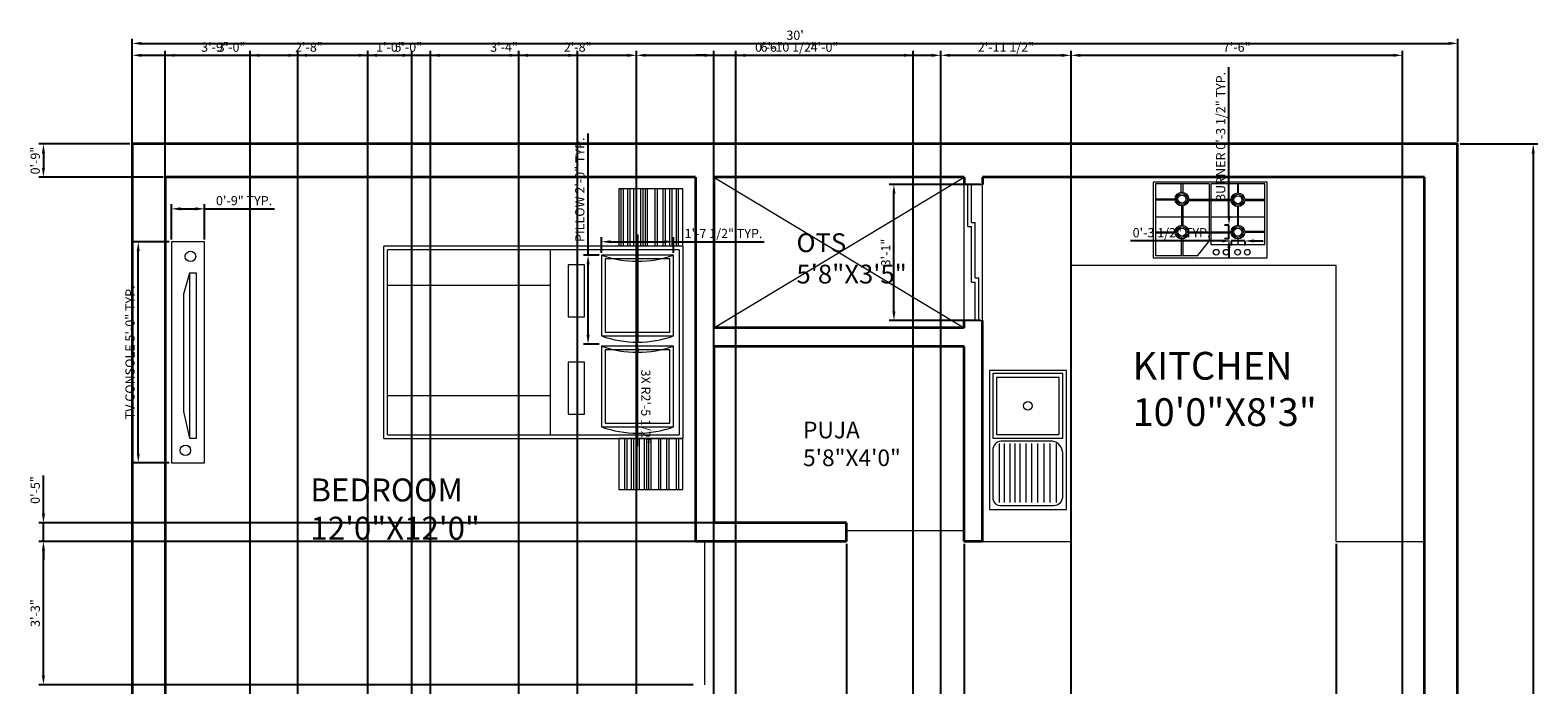
# Model space of a CAD drawing. Units: inches. Extents: x 364 to 777, y 253 to 730.
# Tile 2 of 2: x 364 to 773, y 552 to 730. Entities that reach past the tile are written whole.
import ezdxf

# ---------------------------------------------------------------- set-up
doc = ezdxf.new("R2010")
doc.units = ezdxf.units.IN
for name, color, linetype, lineweight in [('A-ANNO-DIMS', 2, 'Continuous', 18), ('A-AREA-IDEN', 7, 'Continuous', 25), ('A-DOOR', 4, 'Continuous', 18), ('A-EQPM', 8, 'Continuous', 18), ('A-FLOR-CASE', 8, 'Continuous', 18), ('A-FLOR-FIXT', 8, 'Continuous', 18), ('A-FLOR-OPEN', 8, 'Continuous', 13), ('A-FURN', 8, 'Continuous', 18), ('A-GLAZ', 5, 'Continuous', 18), ('A-WALL', 7, 'Continuous', 35)]:
    doc.layers.add(name, color=color, linetype=linetype, lineweight=lineweight)
doc.styles.get("Standard").update_dxf_attribs({"font": 'arial.ttf'})
doc.dimstyles.new('ISO-25', dxfattribs={"dimtxt": 2.5, "dimasz": 2.5, "dimexe": 1.25, "dimexo": 0.625, "dimtad": 1, "dimdec": 0, "dimlunit": 3, "dimtxsty": 'Standard', "dimcen": 2.5, "dimadec": 0, "dimazin": 0, "dimtfac": 1, "dimtdec": 0, "dimtmove": 0, "dimatfit": 3, "dimfxl": 1, "dimarcsym": 0})

# ---------------------------------------------------------------- blocks, each defined once
blk = doc.blocks.new('*D1')
at = {"layer": 'A-ANNO-DIMS', "color": 0, "lineweight": -2, "transparency": 16777216}
for p, q in [((752.34, 699.12), (773.4, 699.12)), ((772.15, 696.62), (772.15, 341.62)), ((752.34, 339.12), (773.4, 339.12))]:
    blk.add_line(p, q, dxfattribs=at)
at = {"layer": 'A-ANNO-DIMS', "color": 0, "transparency": 16777216}
for points in [[(771.73, 696.62), (772.57, 696.62), (772.15, 699.12)], [(771.73, 341.62), (772.57, 341.62), (772.15, 339.12)]]:
    blk.add_solid(points, dxfattribs=at)
at = {"layer": 'Defpoints', "color": 0, "transparency": 16777216}
for p in [(751.71, 699.12), (751.71, 339.12), (772.15, 339.12)]:
    blk.add_point(p, dxfattribs=at)
at = {"layer": 'A-ANNO-DIMS', "color": 0, "transparency": 16777216, "insert": (770.25, 519.12), "char_height": 2.5, "attachment_point": 5, "rotation": 90}
blk.add_mtext("30'", dxfattribs=at)
blk = doc.blocks.new('*D2')
at = {"layer": 'A-ANNO-DIMS', "color": 0, "lineweight": -2, "transparency": 16777216}
for p, q in [((391.61, 699.74), (391.61, 727.71)), ((394.11, 726.46), (749.21, 726.46)), ((751.71, 699.74), (751.71, 727.71))]:
    blk.add_line(p, q, dxfattribs=at)
at = {"layer": 'A-ANNO-DIMS', "color": 0, "transparency": 16777216}
for points in [[(394.11, 726.88), (394.11, 726.04), (391.61, 726.46)], [(749.21, 726.88), (749.21, 726.04), (751.71, 726.46)]]:
    blk.add_solid(points, dxfattribs=at)
at = {"layer": 'Defpoints', "color": 0, "transparency": 16777216}
for p in [(751.71, 726.46), (391.61, 699.12), (751.71, 699.12)]:
    blk.add_point(p, dxfattribs=at)
at = {"layer": 'A-ANNO-DIMS', "color": 0, "transparency": 16777216, "insert": (571.66, 728.36), "char_height": 2.5, "attachment_point": 5}
blk.add_mtext("30'", dxfattribs=at)
blk = doc.blocks.new('TV-CONSOLE-60')
for p, q in [((4.94, 51.53), (3.29, 45.83)), ((3.29, 45.83), (3.29, 13.89)), ((3.29, 13.89), (4.94, 6.65))]:
    blk.add_line(p, q)
for points in [[(9, 0), (9, 60), (0, 60), (0, 0)], [(4.94, 6.65), (6.81, 6.65), (6.81, 51.53), (4.94, 51.53)]]:
    blk.add_lwpolyline(points, close=True)
for centre in [(5.17, 56.08), (3.81, 3.36)]:
    blk.add_circle(centre, 1.42)
blk = doc.blocks.new('BED-PILLOW')
for points in [[(0, 1.69), (19.61, 1.69), (19.61, 23.65), (0, 23.65)], [(1, 2.69), (18.61, 2.69), (18.61, 22.65), (1, 22.65)]]:
    blk.add_lwpolyline(points, close=True)
for centre in [(9.8, 51.22), (9.8, 29.25)]:
    blk.add_arc(centre, 29.25, 250.4189, 289.5811)
blk = doc.blocks.new('COOKTOP-BURNER')
for radius in [1.86, 1.47, 1.08]:
    blk.add_circle((1.86, 1.86), radius)
blk = doc.blocks.new('*D10')
at = {"layer": 'A-ANNO-DIMS', "color": 0, "lineweight": -2, "transparency": 16777216}
for p, q in [((401.65, 672.5), (392.02, 672.5)), ((393.27, 615), (393.27, 670)), ((401.65, 612.5), (392.02, 612.5))]:
    blk.add_line(p, q, dxfattribs=at)
at = {"layer": 'A-ANNO-DIMS', "color": 0, "transparency": 16777216}
for points in [[(392.85, 670), (393.69, 670), (393.27, 672.5)], [(392.85, 615), (393.69, 615), (393.27, 612.5)]]:
    blk.add_solid(points, dxfattribs=at)
at = {"layer": 'Defpoints', "color": 0, "transparency": 16777216}
for p in [(393.27, 672.5), (402.27, 672.5), (402.27, 612.5)]:
    blk.add_point(p, dxfattribs=at)
at = {"layer": 'A-ANNO-DIMS', "color": 0, "transparency": 16777216, "insert": (391.35, 642.5), "char_height": 2.5, "attachment_point": 5, "rotation": 90}
blk.add_mtext('TV CONSOLE 5\'-0" TYP.', dxfattribs=at)
blk = doc.blocks.new('*D11')
at = {"layer": 'A-ANNO-DIMS', "color": 0, "lineweight": -2, "transparency": 16777216}
for p, q in [((402.27, 673.12), (402.27, 682.75)), ((404.77, 681.5), (408.77, 681.5)), ((411.27, 673.12), (411.27, 682.75)), ((411.27, 681.5), (430.26, 681.5))]:
    blk.add_line(p, q, dxfattribs=at)
at = {"layer": 'A-ANNO-DIMS', "color": 0, "transparency": 16777216}
for points in [[(404.77, 681.92), (404.77, 681.08), (402.27, 681.5)], [(408.77, 681.92), (408.77, 681.08), (411.27, 681.5)]]:
    blk.add_solid(points, dxfattribs=at)
at = {"layer": 'Defpoints', "color": 0, "transparency": 16777216}
for p in [(411.27, 681.5), (402.27, 672.5), (411.27, 672.5)]:
    blk.add_point(p, dxfattribs=at)
at = {"layer": 'A-ANNO-DIMS', "color": 0, "transparency": 16777216, "insert": (422.01, 683.4), "char_height": 2.5, "attachment_point": 5}
blk.add_mtext('0\'-9" TYP.', dxfattribs=at)
blk = doc.blocks.new('*D12')
at = {"layer": 'A-ANNO-DIMS', "color": 0, "lineweight": -2, "transparency": 16777216}
for p, q in [((515.44, 668.92), (515.44, 701.96)), ((518.45, 668.92), (514.19, 668.92)), ((515.44, 647.21), (515.44, 666.42)), ((518.45, 644.71), (514.19, 644.71))]:
    blk.add_line(p, q, dxfattribs=at)
at = {"layer": 'A-ANNO-DIMS', "color": 0, "transparency": 16777216}
for points in [[(515.02, 666.42), (515.86, 666.42), (515.44, 668.92)], [(515.02, 647.21), (515.86, 647.21), (515.44, 644.71)]]:
    blk.add_solid(points, dxfattribs=at)
at = {"layer": 'Defpoints', "color": 0, "transparency": 16777216}
for p in [(515.44, 668.92), (519.07, 668.92), (519.07, 644.71)]:
    blk.add_point(p, dxfattribs=at)
at = {"layer": 'A-ANNO-DIMS', "color": 0, "transparency": 16777216, "insert": (513.52, 686.69), "char_height": 2.5, "attachment_point": 5, "rotation": 90}
blk.add_mtext('PILLOW 2\'-0" TYP.', dxfattribs=at)
blk = doc.blocks.new('*D13')
at = {"layer": 'A-ANNO-DIMS', "color": 0, "lineweight": -2, "transparency": 16777216}
for p, q in [((519.07, 669.55), (519.07, 673.81)), ((521.57, 672.56), (536.18, 672.56)), ((538.68, 669.55), (538.68, 673.81)), ((538.68, 672.56), (563.26, 672.56))]:
    blk.add_line(p, q, dxfattribs=at)
at = {"layer": 'A-ANNO-DIMS', "color": 0, "transparency": 16777216}
for points in [[(521.57, 672.97), (521.57, 672.14), (519.07, 672.56)], [(536.18, 672.97), (536.18, 672.14), (538.68, 672.56)]]:
    blk.add_solid(points, dxfattribs=at)
at = {"layer": 'Defpoints', "color": 0, "transparency": 16777216}
for p in [(538.68, 672.56), (519.07, 668.92), (538.68, 668.92)]:
    blk.add_point(p, dxfattribs=at)
at = {"layer": 'A-ANNO-DIMS', "color": 0, "transparency": 16777216, "insert": (552.22, 674.47), "char_height": 2.5, "attachment_point": 5}
blk.add_mtext('1\'-7 1/2" TYP.', dxfattribs=at)
blk = doc.blocks.new('*D14')
at = {"layer": 'A-ANNO-DIMS', "color": 0, "lineweight": -2, "transparency": 16777216}
for p, q in [((689.51, 679.55), (689.51, 719.97)), ((689.44, 677.05), (688.26, 677.05)), ((689.51, 673.33), (689.51, 677.05)), ((689.44, 673.33), (688.26, 673.33)), ((689.51, 670.83), (689.51, 668.33))]:
    blk.add_line(p, q, dxfattribs=at)
at = {"layer": 'A-ANNO-DIMS', "color": 0, "transparency": 16777216}
for points in [[(689.09, 679.55), (689.93, 679.55), (689.51, 677.05)], [(689.09, 670.83), (689.93, 670.83), (689.51, 673.33)]]:
    blk.add_solid(points, dxfattribs=at)
at = {"layer": 'Defpoints', "color": 0, "transparency": 16777216}
for p in [(689.51, 677.05), (690.07, 677.05), (690.07, 673.33)]:
    blk.add_point(p, dxfattribs=at)
at = {"layer": 'A-ANNO-DIMS', "color": 0, "transparency": 16777216, "insert": (687.59, 701.01), "char_height": 2.5, "attachment_point": 5, "rotation": 90}
blk.add_mtext('BURNER 0\'-3 1/2" TYP.', dxfattribs=at)
blk = doc.blocks.new('*D15')
at = {"layer": 'A-ANNO-DIMS', "color": 0, "lineweight": -2, "transparency": 16777216}
for p, q in [((687.57, 672.77), (662.75, 672.77)), ((693.78, 672.77), (690.07, 672.77)), ((690.07, 672.71), (690.07, 671.52)), ((693.78, 672.71), (693.78, 671.52)), ((696.28, 672.77), (698.78, 672.77))]:
    blk.add_line(p, q, dxfattribs=at)
at = {"layer": 'A-ANNO-DIMS', "color": 0, "transparency": 16777216}
for points in [[(687.57, 673.19), (687.57, 672.36), (690.07, 672.77)], [(696.28, 673.19), (696.28, 672.36), (693.78, 672.77)]]:
    blk.add_solid(points, dxfattribs=at)
at = {"layer": 'Defpoints', "color": 0, "transparency": 16777216}
for p in [(690.07, 673.33), (690.07, 672.77), (693.78, 673.33)]:
    blk.add_point(p, dxfattribs=at)
at = {"layer": 'A-ANNO-DIMS', "color": 0, "transparency": 16777216, "insert": (673.91, 674.69), "char_height": 2.5, "attachment_point": 5}
blk.add_mtext('0\'-3 1/2" TYP.', dxfattribs=at)
blk = doc.blocks.new('*D18')
at = {"layer": 'A-ANNO-DIMS', "color": 0, "lineweight": -2, "transparency": 16777216}
for p, q in [((621.99, 688.12), (597.26, 688.12)), ((598.51, 653.62), (598.51, 685.62)), ((621.99, 651.12), (597.26, 651.12))]:
    blk.add_line(p, q, dxfattribs=at)
at = {"layer": 'A-ANNO-DIMS', "color": 0, "transparency": 16777216}
for points in [[(598.1, 685.62), (598.93, 685.62), (598.51, 688.12)], [(598.1, 653.62), (598.93, 653.62), (598.51, 651.12)]]:
    blk.add_solid(points, dxfattribs=at)
at = {"layer": 'Defpoints', "color": 0, "transparency": 16777216}
for p in [(598.51, 688.12), (622.61, 688.12), (622.61, 651.12)]:
    blk.add_point(p, dxfattribs=at)
at = {"layer": 'A-ANNO-DIMS', "color": 0, "transparency": 16777216, "insert": (596.61, 669.62), "char_height": 2.5, "attachment_point": 5, "rotation": 90}
blk.add_mtext('3\'-1"', dxfattribs=at)
blk = doc.blocks.new('*D20')
at = {"layer": 'A-ANNO-DIMS', "color": 0, "lineweight": -2, "transparency": 16777216}
for p, q in [((543.99, 591.12), (366.26, 591.12)), ((367.51, 554.62), (367.51, 588.62)), ((543.99, 552.12), (366.26, 552.12))]:
    blk.add_line(p, q, dxfattribs=at)
at = {"layer": 'A-ANNO-DIMS', "color": 0, "transparency": 16777216}
for points in [[(367.1, 588.62), (367.93, 588.62), (367.51, 591.12)], [(367.1, 554.62), (367.93, 554.62), (367.51, 552.12)]]:
    blk.add_solid(points, dxfattribs=at)
at = {"layer": 'Defpoints', "color": 0, "transparency": 16777216}
for p in [(367.51, 591.12), (544.61, 591.12), (544.61, 552.12)]:
    blk.add_point(p, dxfattribs=at)
at = {"layer": 'A-ANNO-DIMS', "color": 0, "transparency": 16777216, "insert": (365.61, 571.62), "char_height": 2.5, "attachment_point": 5, "rotation": 90}
blk.add_mtext('3\'-3"', dxfattribs=at)
blk = doc.blocks.new('*D21')
at = {"layer": 'A-ANNO-DIMS', "color": 0, "lineweight": -2, "transparency": 16777216}
for p, q in [((391.61, 339.74), (391.61, 724.47)), ((394.11, 723.22), (434.11, 723.22)), ((436.61, 339.74), (436.61, 724.47))]:
    blk.add_line(p, q, dxfattribs=at)
at = {"layer": 'A-ANNO-DIMS', "color": 0, "transparency": 16777216}
for points in [[(394.11, 723.64), (394.11, 722.8), (391.61, 723.22)], [(434.11, 723.64), (434.11, 722.8), (436.61, 723.22)]]:
    blk.add_solid(points, dxfattribs=at)
at = {"layer": 'Defpoints', "color": 0, "transparency": 16777216}
for p in [(436.61, 723.22), (391.61, 339.12), (436.61, 339.12)]:
    blk.add_point(p, dxfattribs=at)
at = {"layer": 'A-ANNO-DIMS', "color": 0, "transparency": 16777216, "insert": (414.11, 725.12), "char_height": 2.5, "attachment_point": 5}
blk.add_mtext('3\'-9"', dxfattribs=at)
blk = doc.blocks.new('*D22')
at = {"layer": 'A-ANNO-DIMS', "color": 0, "lineweight": -2, "transparency": 16777216}
for p, q in [((436.61, 348.74), (436.61, 724.47)), ((439.11, 723.22), (494.11, 723.22)), ((496.61, 348.74), (496.61, 724.47))]:
    blk.add_line(p, q, dxfattribs=at)
at = {"layer": 'A-ANNO-DIMS', "color": 0, "transparency": 16777216}
for points in [[(439.11, 723.64), (439.11, 722.8), (436.61, 723.22)], [(494.11, 723.64), (494.11, 722.8), (496.61, 723.22)]]:
    blk.add_solid(points, dxfattribs=at)
at = {"layer": 'Defpoints', "color": 0, "transparency": 16777216}
for p in [(496.61, 723.22), (436.61, 348.12), (496.61, 348.12)]:
    blk.add_point(p, dxfattribs=at)
at = {"layer": 'A-ANNO-DIMS', "color": 0, "transparency": 16777216, "insert": (466.61, 725.12), "char_height": 2.5, "attachment_point": 5}
blk.add_mtext('5\'-0"', dxfattribs=at)
blk = doc.blocks.new('*D23')
at = {"layer": 'A-ANNO-DIMS', "color": 0, "lineweight": -2, "transparency": 16777216}
for p, q in [((496.61, 339.74), (496.61, 724.47)), ((499.11, 723.22), (526.11, 723.22)), ((528.61, 339.74), (528.61, 724.47))]:
    blk.add_line(p, q, dxfattribs=at)
at = {"layer": 'A-ANNO-DIMS', "color": 0, "transparency": 16777216}
for points in [[(499.11, 723.64), (499.11, 722.8), (496.61, 723.22)], [(526.11, 723.64), (526.11, 722.8), (528.61, 723.22)]]:
    blk.add_solid(points, dxfattribs=at)
at = {"layer": 'Defpoints', "color": 0, "transparency": 16777216}
for p in [(528.61, 723.22), (496.61, 339.12), (528.61, 339.12)]:
    blk.add_point(p, dxfattribs=at)
at = {"layer": 'A-ANNO-DIMS', "color": 0, "transparency": 16777216, "insert": (512.61, 725.12), "char_height": 2.5, "attachment_point": 5}
blk.add_mtext('2\'-8"', dxfattribs=at)
blk = doc.blocks.new('*D24')
at = {"layer": 'A-ANNO-DIMS', "color": 0, "lineweight": -2, "transparency": 16777216}
for p, q in [((528.61, 348.74), (528.61, 724.47)), ((531.11, 723.22), (608.76, 723.22)), ((611.26, 348.74), (611.26, 724.47))]:
    blk.add_line(p, q, dxfattribs=at)
at = {"layer": 'A-ANNO-DIMS', "color": 0, "transparency": 16777216}
for points in [[(531.11, 723.64), (531.11, 722.8), (528.61, 723.22)], [(608.76, 723.64), (608.76, 722.8), (611.26, 723.22)]]:
    blk.add_solid(points, dxfattribs=at)
at = {"layer": 'Defpoints', "color": 0, "transparency": 16777216}
for p in [(611.26, 723.22), (528.61, 348.12), (611.26, 348.12)]:
    blk.add_point(p, dxfattribs=at)
at = {"layer": 'A-ANNO-DIMS', "color": 0, "transparency": 16777216, "insert": (569.94, 725.14), "char_height": 2.5, "attachment_point": 5}
blk.add_mtext('6\'-10 1/2"', dxfattribs=at)
blk = doc.blocks.new('*D25')
at = {"layer": 'A-ANNO-DIMS', "color": 0, "lineweight": -2, "transparency": 16777216}
for p, q in [((611.26, 339.74), (611.26, 724.47)), ((613.76, 723.22), (644.11, 723.22)), ((646.61, 339.74), (646.61, 724.47))]:
    blk.add_line(p, q, dxfattribs=at)
at = {"layer": 'A-ANNO-DIMS', "color": 0, "transparency": 16777216}
for points in [[(613.76, 723.64), (613.76, 722.8), (611.26, 723.22)], [(644.11, 723.64), (644.11, 722.8), (646.61, 723.22)]]:
    blk.add_solid(points, dxfattribs=at)
at = {"layer": 'Defpoints', "color": 0, "transparency": 16777216}
for p in [(646.61, 723.22), (611.26, 339.12), (646.61, 339.12)]:
    blk.add_point(p, dxfattribs=at)
at = {"layer": 'A-ANNO-DIMS', "color": 0, "transparency": 16777216, "insert": (628.94, 725.14), "char_height": 2.5, "attachment_point": 5}
blk.add_mtext('2\'-11 1/2"', dxfattribs=at)
blk = doc.blocks.new('*D26')
at = {"layer": 'A-ANNO-DIMS', "color": 0, "lineweight": -2, "transparency": 16777216}
for p, q in [((646.61, 348.74), (646.61, 724.47)), ((649.11, 723.22), (734.11, 723.22)), ((736.61, 348.74), (736.61, 724.47))]:
    blk.add_line(p, q, dxfattribs=at)
at = {"layer": 'A-ANNO-DIMS', "color": 0, "transparency": 16777216}
for points in [[(649.11, 723.64), (649.11, 722.8), (646.61, 723.22)], [(734.11, 723.64), (734.11, 722.8), (736.61, 723.22)]]:
    blk.add_solid(points, dxfattribs=at)
at = {"layer": 'Defpoints', "color": 0, "transparency": 16777216}
for p in [(736.61, 723.22), (646.61, 348.12), (736.61, 348.12)]:
    blk.add_point(p, dxfattribs=at)
at = {"layer": 'A-ANNO-DIMS', "color": 0, "transparency": 16777216, "insert": (691.61, 725.12), "char_height": 2.5, "attachment_point": 5}
blk.add_mtext('7\'-6"', dxfattribs=at)
blk = doc.blocks.new('*D27')
at = {"layer": 'A-ANNO-DIMS', "color": 0, "lineweight": -2, "transparency": 16777216}
for p, q in [((390.99, 699.12), (366.26, 699.12)), ((367.51, 696.62), (367.51, 692.62)), ((399.99, 690.12), (366.26, 690.12))]:
    blk.add_line(p, q, dxfattribs=at)
at = {"layer": 'A-ANNO-DIMS', "color": 0, "transparency": 16777216}
for points in [[(367.1, 696.62), (367.93, 696.62), (367.51, 699.12)], [(367.1, 692.62), (367.93, 692.62), (367.51, 690.12)]]:
    blk.add_solid(points, dxfattribs=at)
at = {"layer": 'Defpoints', "color": 0, "transparency": 16777216}
for p in [(391.61, 699.12), (367.51, 690.12), (400.61, 690.12)]:
    blk.add_point(p, dxfattribs=at)
at = {"layer": 'A-ANNO-DIMS', "color": 0, "transparency": 16777216, "insert": (365.61, 694.62), "char_height": 2.5, "attachment_point": 5, "rotation": 90}
blk.add_mtext('0\'-9"', dxfattribs=at)
blk = doc.blocks.new('*D28')
at = {"layer": 'A-ANNO-DIMS', "color": 0, "lineweight": -2, "transparency": 16777216}
for p, q in [((367.51, 598.62), (367.51, 609.01)), ((584.99, 596.12), (366.26, 596.12)), ((367.51, 591.12), (367.51, 596.12)), ((584.99, 591.12), (366.26, 591.12)), ((367.51, 588.62), (367.51, 586.12))]:
    blk.add_line(p, q, dxfattribs=at)
at = {"layer": 'A-ANNO-DIMS', "color": 0, "transparency": 16777216}
for points in [[(367.1, 598.62), (367.93, 598.62), (367.51, 596.12)], [(367.1, 588.62), (367.93, 588.62), (367.51, 591.12)]]:
    blk.add_solid(points, dxfattribs=at)
at = {"layer": 'Defpoints', "color": 0, "transparency": 16777216}
for p in [(367.51, 596.12), (585.61, 596.12), (585.61, 591.12)]:
    blk.add_point(p, dxfattribs=at)
at = {"layer": 'A-ANNO-DIMS', "color": 0, "transparency": 16777216, "insert": (365.61, 605.07), "char_height": 2.5, "attachment_point": 5, "rotation": 90}
blk.add_mtext('0\'-5"', dxfattribs=at)
blk = doc.blocks.new('*D29')
at = {"layer": 'A-ANNO-DIMS', "color": 0, "lineweight": -2, "transparency": 16777216}
for p, q in [((455.62, 541.74), (455.62, 724.47)), ((458.12, 723.22), (465.11, 723.22)), ((467.61, 541.74), (467.61, 724.47))]:
    blk.add_line(p, q, dxfattribs=at)
at = {"layer": 'A-ANNO-DIMS', "color": 0, "transparency": 16777216}
for points in [[(458.12, 723.64), (458.12, 722.8), (455.62, 723.22)], [(465.11, 723.64), (465.11, 722.8), (467.61, 723.22)]]:
    blk.add_solid(points, dxfattribs=at)
at = {"layer": 'Defpoints', "color": 0, "transparency": 16777216}
for p in [(467.61, 723.22), (455.62, 541.12), (467.61, 541.12)]:
    blk.add_point(p, dxfattribs=at)
at = {"layer": 'A-ANNO-DIMS', "color": 0, "transparency": 16777216, "insert": (461.62, 725.12), "char_height": 2.5, "attachment_point": 5}
blk.add_mtext('1\'-0"', dxfattribs=at)
blk = doc.blocks.new('*D30')
at = {"layer": 'A-ANNO-DIMS', "color": 0, "lineweight": -2, "transparency": 16777216}
for p, q in [((423.62, 546.74), (423.62, 724.47)), ((426.12, 723.22), (453.12, 723.22)), ((455.62, 546.74), (455.62, 724.47))]:
    blk.add_line(p, q, dxfattribs=at)
at = {"layer": 'A-ANNO-DIMS', "color": 0, "transparency": 16777216}
for points in [[(426.12, 723.64), (426.12, 722.8), (423.62, 723.22)], [(453.12, 723.64), (453.12, 722.8), (455.62, 723.22)]]:
    blk.add_solid(points, dxfattribs=at)
at = {"layer": 'Defpoints', "color": 0, "transparency": 16777216}
for p in [(455.62, 723.22), (423.62, 546.12), (455.62, 546.12)]:
    blk.add_point(p, dxfattribs=at)
at = {"layer": 'A-ANNO-DIMS', "color": 0, "transparency": 16777216, "insert": (439.62, 725.12), "char_height": 2.5, "attachment_point": 5}
blk.add_mtext('2\'-8"', dxfattribs=at)
blk = doc.blocks.new('*D31')
at = {"layer": 'A-ANNO-DIMS', "color": 0, "lineweight": -2, "transparency": 16777216}
for p, q in [((585.61, 590.49), (585.61, 293.23)), ((617.61, 590.49), (617.61, 293.23)), ((588.11, 294.48), (615.11, 294.48))]:
    blk.add_line(p, q, dxfattribs=at)
at = {"layer": 'A-ANNO-DIMS', "color": 0, "transparency": 16777216}
for points in [[(588.11, 294.9), (588.11, 294.06), (585.61, 294.48)], [(615.11, 294.9), (615.11, 294.06), (617.61, 294.48)]]:
    blk.add_solid(points, dxfattribs=at)
at = {"layer": 'Defpoints', "color": 0, "transparency": 16777216}
for p in [(585.61, 591.12), (617.61, 591.12), (617.61, 294.48)]:
    blk.add_point(p, dxfattribs=at)
at = {"layer": 'A-ANNO-DIMS', "color": 0, "transparency": 16777216, "insert": (601.61, 296.38), "char_height": 2.5, "attachment_point": 5}
blk.add_mtext('2\'-8"', dxfattribs=at)
blk = doc.blocks.new('*D32')
at = {"layer": 'A-ANNO-DIMS', "color": 0, "lineweight": -2, "transparency": 16777216}
for p, q in [((555.61, 473.74), (555.61, 724.47)), ((558.11, 723.22), (601.21, 723.22)), ((603.71, 473.74), (603.71, 724.47))]:
    blk.add_line(p, q, dxfattribs=at)
at = {"layer": 'A-ANNO-DIMS', "color": 0, "transparency": 16777216}
for points in [[(558.11, 723.64), (558.11, 722.8), (555.61, 723.22)], [(601.21, 723.64), (601.21, 722.8), (603.71, 723.22)]]:
    blk.add_solid(points, dxfattribs=at)
at = {"layer": 'Defpoints', "color": 0, "transparency": 16777216}
for p in [(603.71, 723.22), (555.61, 473.12), (603.71, 473.12)]:
    blk.add_point(p, dxfattribs=at)
at = {"layer": 'A-ANNO-DIMS', "color": 0, "transparency": 16777216, "insert": (579.66, 725.12), "char_height": 2.5, "attachment_point": 5}
blk.add_mtext('4\'-0"', dxfattribs=at)
blk = doc.blocks.new('*D34')
at = {"layer": 'A-ANNO-DIMS', "color": 0, "lineweight": -2, "transparency": 16777216}
for p, q in [((718.61, 590.49), (718.61, 293.23)), ((742.61, 590.49), (742.61, 293.23)), ((721.11, 294.48), (740.11, 294.48))]:
    blk.add_line(p, q, dxfattribs=at)
at = {"layer": 'A-ANNO-DIMS', "color": 0, "transparency": 16777216}
for points in [[(721.11, 294.9), (721.11, 294.06), (718.61, 294.48)], [(740.11, 294.9), (740.11, 294.06), (742.61, 294.48)]]:
    blk.add_solid(points, dxfattribs=at)
at = {"layer": 'Defpoints', "color": 0, "transparency": 16777216}
for p in [(718.61, 591.12), (742.61, 591.12), (742.61, 294.48)]:
    blk.add_point(p, dxfattribs=at)
at = {"layer": 'A-ANNO-DIMS', "color": 0, "transparency": 16777216, "insert": (730.61, 296.38), "char_height": 2.5, "attachment_point": 5}
blk.add_mtext('2\'-0"', dxfattribs=at)
blk = doc.blocks.new('*D35')
at = {"layer": 'A-ANNO-DIMS', "color": 0, "lineweight": -2, "transparency": 16777216}
for p, q in [((400.61, 428.74), (400.61, 724.47)), ((403.11, 723.22), (434.11, 723.22)), ((436.61, 428.74), (436.61, 724.47))]:
    blk.add_line(p, q, dxfattribs=at)
at = {"layer": 'A-ANNO-DIMS', "color": 0, "transparency": 16777216}
for points in [[(403.11, 723.64), (403.11, 722.8), (400.61, 723.22)], [(434.11, 723.64), (434.11, 722.8), (436.61, 723.22)]]:
    blk.add_solid(points, dxfattribs=at)
at = {"layer": 'Defpoints', "color": 0, "transparency": 16777216}
for p in [(436.61, 723.22), (400.61, 428.12), (436.61, 428.12)]:
    blk.add_point(p, dxfattribs=at)
at = {"layer": 'A-ANNO-DIMS', "color": 0, "transparency": 16777216, "insert": (418.61, 725.12), "char_height": 2.5, "attachment_point": 5}
blk.add_mtext('3\'-0"', dxfattribs=at)
blk = doc.blocks.new('*D36')
at = {"layer": 'A-ANNO-DIMS', "color": 0, "lineweight": -2, "transparency": 16777216}
for p, q in [((472.61, 473.74), (472.61, 724.47)), ((475.11, 723.22), (510.11, 723.22)), ((512.61, 473.74), (512.61, 724.47))]:
    blk.add_line(p, q, dxfattribs=at)
at = {"layer": 'A-ANNO-DIMS', "color": 0, "transparency": 16777216}
for points in [[(475.11, 723.64), (475.11, 722.8), (472.61, 723.22)], [(510.11, 723.64), (510.11, 722.8), (512.61, 723.22)]]:
    blk.add_solid(points, dxfattribs=at)
at = {"layer": 'Defpoints', "color": 0, "transparency": 16777216}
for p in [(512.61, 723.22), (472.61, 473.12), (512.61, 473.12)]:
    blk.add_point(p, dxfattribs=at)
at = {"layer": 'A-ANNO-DIMS', "color": 0, "transparency": 16777216, "insert": (492.61, 725.12), "char_height": 2.5, "attachment_point": 5}
blk.add_mtext('3\'-4"', dxfattribs=at)
blk = doc.blocks.new('*D37')
at = {"layer": 'A-ANNO-DIMS', "color": 0, "lineweight": -2, "transparency": 16777216}
for p, q in [((547.11, 723.22), (544.61, 723.22)), ((549.61, 473.74), (549.61, 724.47)), ((549.61, 723.22), (555.61, 723.22)), ((555.61, 473.74), (555.61, 724.47)), ((558.11, 723.22), (568.51, 723.22))]:
    blk.add_line(p, q, dxfattribs=at)
at = {"layer": 'A-ANNO-DIMS', "color": 0, "transparency": 16777216}
for points in [[(547.11, 723.64), (547.11, 722.8), (549.61, 723.22)], [(558.11, 723.64), (558.11, 722.8), (555.61, 723.22)]]:
    blk.add_solid(points, dxfattribs=at)
at = {"layer": 'Defpoints', "color": 0, "transparency": 16777216}
for p in [(555.61, 723.22), (549.61, 473.12), (555.61, 473.12)]:
    blk.add_point(p, dxfattribs=at)
at = {"layer": 'A-ANNO-DIMS', "color": 0, "transparency": 16777216, "insert": (564.56, 725.12), "char_height": 2.5, "attachment_point": 5}
blk.add_mtext('0\'-6"', dxfattribs=at)
blk = doc.blocks.new('*D38')
at = {"layer": 'A-ANNO-DIMS', "color": 0, "lineweight": -2, "transparency": 16777216}
for p, q in [((528.88, 674.52), (528.88, 645.27)), ((528.88, 616.98), (528.88, 642.77))]:
    blk.add_line(p, q, dxfattribs=at)
at = {"layer": 'A-ANNO-DIMS', "color": 0, "transparency": 16777216}
blk.add_solid([(529.29, 642.77), (528.46, 642.77), (528.88, 645.27)], dxfattribs=at)
at = {"layer": 'Defpoints', "color": 0, "transparency": 16777216}
for p in [(528.88, 674.52), (528.88, 645.27)]:
    blk.add_point(p, dxfattribs=at)
at = {"layer": 'A-ANNO-DIMS', "color": 0, "transparency": 16777216, "insert": (530.79, 627.72), "char_height": 2.5, "attachment_point": 5, "rotation": 270.0005}
blk.add_mtext('3X R2\'-5 1/2"', dxfattribs=at)

msp = doc.modelspace()

# ---------------------------------------------------------------- linework, layer by layer
at = {"layer": 'A-DOOR'}
for p, q in [((617.61, 593.95), (585.61, 593.95)), ((547.11, 552.12), (547.11, 591.12))]:
    msp.add_line(p, q, dxfattribs=at)
at = {"layer": 'A-EQPM'}
for p, q in [((668.92, 688.82), (668.92, 668.16)), ((668.92, 688.82), (699.85, 688.82)), ((684.09, 688.26), (669.57, 688.26)), ((669.57, 688.26), (669.57, 668.8)), ((676.55, 686.01), (676.55, 688.25)), ((677.05, 685.99), (677.05, 688.23)), ((684.09, 688.26), (684.09, 672.69)), ((684.57, 688.25), (684.57, 671.82)), ((699.22, 688.25), (684.57, 688.25)), ((691.92, 685.83), (691.92, 688.25)), ((692.14, 685.82), (692.14, 688.24)), ((699.22, 671.82), (699.22, 688.25)), ((699.85, 668.16), (699.85, 688.82)), ((674.87, 684.16), (669.57, 684.16)), ((678.58, 684.16), (690.08, 684.16)), ((693.77, 684.16), (699.22, 684.16)), ((674.9, 683.83), (669.6, 683.83)), ((676.57, 682.31), (676.57, 677.04)), ((676.96, 682.32), (676.96, 677.03)), ((678.54, 683.76), (690.08, 683.76)), ((691.92, 677.05), (691.92, 682.11)), ((692.13, 677.04), (692.13, 682.1)), ((693.77, 683.79), (699.22, 683.79)), ((684.09, 679.26), (669.57, 679.26)), ((699.22, 679.26), (684.57, 679.26)), ((674.87, 675.19), (669.57, 675.19)), ((674.9, 674.85), (669.6, 674.85)), ((676.48, 673.35), (676.48, 668.8)), ((676.99, 673.35), (676.99, 668.8)), ((678.57, 674.98), (690.08, 674.98)), ((678.58, 675.22), (690.07, 675.22)), ((681.08, 668.8), (684.09, 672.69)), ((684.57, 671.82), (699.22, 671.82)), ((691.92, 673.33), (691.92, 671.82)), ((693.77, 675.41), (699.21, 675.41)), ((693.78, 675.19), (699.22, 675.19)), ((668.92, 668.16), (699.85, 668.16)), ((669.57, 668.8), (678.63, 668.8)), ((678.63, 668.8), (681.08, 668.8))]:
    msp.add_line(p, q, dxfattribs=at)
for centre in [(686.05, 669.71), (688.76, 669.71), (691.85, 669.71), (694.49, 669.71)]:
    msp.add_circle(centre, 0.764, dxfattribs=at)
at = {"layer": 'A-FLOR-CASE'}
for p, q in [((646.61, 591.12), (646.61, 666.12)), ((718.61, 666.12), (646.61, 666.12)), ((718.61, 591.12), (718.61, 666.12)), ((622.61, 591.12), (646.61, 591.12)), ((718.61, 591.12), (742.61, 591.12))]:
    msp.add_line(p, q, dxfattribs=at)
at = {"layer": 'A-FLOR-FIXT'}
for p, q in [((644.36, 636.7), (625.35, 636.7)), ((625.35, 636.7), (625.35, 619.19)), ((644.36, 619.19), (644.36, 636.7)), ((625.35, 619.19), (644.36, 619.19)), ((641.59, 618.37), (627.51, 618.37)), ((625.35, 615.91), (625.35, 602.6)), ((627.19, 601.71), (627.19, 617.69)), ((628.51, 601.71), (628.51, 617.69)), ((630.06, 601.71), (630.06, 617.69)), ((631.45, 601.71), (631.45, 617.69)), ((632.8, 601.71), (632.8, 617.69)), ((634.45, 601.71), (634.45, 617.69)), ((635.93, 601.71), (635.93, 617.69)), ((637.55, 601.71), (637.55, 617.69)), ((639.27, 601.71), (639.27, 617.69)), ((640.95, 601.71), (640.95, 617.69)), ((642.63, 601.71), (642.63, 617.69)), ((644.36, 603.16), (644.36, 615.06)), ((627.43, 600.87), (641.86, 600.87))]:
    msp.add_line(p, q, dxfattribs=at)
for points in [[(624.46, 599.79), (645.41, 599.79), (645.41, 637.58), (624.46, 637.58)], [(643.36, 620.2), (643.36, 635.69), (626.36, 635.69), (626.36, 620.2)]]:
    msp.add_lwpolyline(points, close=True, dxfattribs=at)
msp.add_circle((634.86, 627.94), 1.19, dxfattribs=at)
for centre, radius, start, end in [((627.83, 615.91), 2.48, 97.3953, 180), ((641, 615.06), 3.36, 0, 79.8896), ((627.43, 602.98), 2.11, 190.2616, 270), ((641.86, 603.37), 2.51, 270, 4.7981)]:
    msp.add_arc(centre, radius, start, end, dxfattribs=at)
at = {"layer": 'A-FLOR-OPEN'}
for p, q in [((549.61, 649.12), (617.61, 690.12)), ((549.61, 690.12), (617.61, 649.12))]:
    msp.add_line(p, q, dxfattribs=at)
at = {"layer": 'A-FURN'}
for p, q in [((541.16, 686.96), (523.81, 686.96)), ((523.81, 686.96), (523.81, 671.35)), ((524.36, 686.96), (524.36, 671.35)), ((524.98, 686.96), (524.98, 671.35)), ((526.17, 686.96), (526.17, 671.35)), ((526.79, 686.96), (526.79, 671.35)), ((527.75, 686.96), (527.75, 671.35)), ((528.37, 686.96), (528.37, 671.35)), ((529.72, 686.96), (529.72, 671.35)), ((530.33, 686.96), (530.33, 671.35)), ((530.91, 686.96), (530.91, 671.35)), ((531.53, 686.96), (531.53, 671.35)), ((533.57, 686.96), (533.57, 671.35)), ((534.19, 686.96), (534.19, 671.35)), ((535.77, 686.96), (535.77, 671.35)), ((536.39, 686.96), (536.39, 671.35)), ((537.57, 686.96), (537.57, 671.35)), ((538.18, 686.96), (538.18, 671.35)), ((539.32, 686.96), (539.32, 671.35)), ((539.94, 686.96), (539.94, 671.35)), ((541.16, 671.35), (541.16, 686.96)), ((541.16, 671.35), (459.99, 671.35)), ((459.99, 619.05), (459.99, 671.35)), ((540.16, 670.35), (460.99, 670.35)), ((460.99, 620.05), (460.99, 670.35)), ((505.27, 620.05), (505.27, 670.35)), ((540.16, 670.35), (540.16, 620.05)), ((541.16, 671.35), (541.16, 619.05)), ((460.99, 660.74), (505.27, 660.74)), ((460.99, 630.77), (505.27, 630.77)), ((459.99, 619.05), (541.16, 619.05)), ((460.99, 620.05), (540.16, 620.05)), ((541.16, 619.05), (523.81, 619.05)), ((523.81, 619.05), (523.81, 605.19)), ((525.31, 619.05), (525.31, 605.19)), ((525.93, 619.05), (525.93, 605.19)), ((527.12, 619.05), (527.12, 605.19)), ((527.74, 619.05), (527.74, 605.19)), ((528.7, 619.05), (528.7, 605.19)), ((529.32, 619.05), (529.32, 605.19)), ((530.67, 619.05), (530.67, 605.19)), ((531.29, 619.05), (531.29, 605.19)), ((531.87, 619.05), (531.87, 605.19)), ((532.48, 619.05), (532.48, 605.19)), ((534.53, 619.05), (534.53, 605.19)), ((535.14, 619.05), (535.14, 605.19)), ((536.72, 619.05), (536.72, 605.19)), ((537.34, 619.05), (537.34, 605.19)), ((539.38, 619.05), (539.38, 605.19)), ((540, 619.05), (540, 605.19)), ((541.16, 605.19), (541.16, 619.05)), ((523.81, 605.19), (541.16, 605.19))]:
    msp.add_line(p, q, dxfattribs=at)
for points in [[(510.07, 652.12), (514.49, 652.12), (514.49, 666.28), (510.07, 666.28)], [(510.07, 625.67), (514.49, 625.67), (514.49, 639.83), (510.07, 639.83)]]:
    msp.add_lwpolyline(points, close=True, dxfattribs=at)
at = {"layer": 'A-GLAZ'}
for p, q in [((617.61, 688.12), (622.61, 688.12)), ((617.61, 651.12), (617.61, 688.12)), ((617.61, 688.12), (622.61, 688.12)), ((618.61, 676.7), (618.61, 688.12)), ((619.61, 677.76), (619.61, 688.12)), ((622.61, 651.12), (622.61, 688.12)), ((618.61, 676.7), (619.61, 676.7)), ((619.61, 677.76), (620.61, 677.76)), ((619.61, 661.56), (619.61, 676.7)), ((620.61, 662.71), (620.61, 677.76)), ((619.61, 661.56), (620.61, 661.56)), ((620.61, 662.71), (621.61, 662.71)), ((620.61, 651.12), (620.61, 661.56)), ((621.61, 651.12), (621.61, 662.71)), ((617.61, 651.12), (622.61, 651.12))]:
    msp.add_line(p, q, dxfattribs=at)
at = {"layer": 'A-WALL'}
for p, q in [((400.61, 690.12), (400.61, 546.12)), ((544.61, 690.12), (400.61, 690.12)), ((544.61, 690.12), (544.61, 591.12)), ((549.61, 690.12), (549.61, 649.12)), ((617.61, 690.12), (549.61, 690.12)), ((617.61, 690.12), (617.61, 688.12)), ((742.61, 690.12), (622.61, 690.12)), ((622.61, 690.12), (622.61, 688.12)), ((742.61, 473.12), (742.61, 690.12)), ((617.61, 649.12), (617.61, 651.12)), ((622.61, 591.12), (622.61, 651.12)), ((617.61, 649.12), (549.61, 649.12)), ((617.61, 644.12), (549.61, 644.12)), ((549.61, 644.12), (549.61, 596.12)), ((617.61, 591.12), (617.61, 644.12)), ((585.61, 596.12), (549.61, 596.12)), ((585.61, 591.12), (585.61, 596.12)), ((585.61, 591.12), (544.61, 591.12)), ((622.61, 591.12), (617.61, 591.12))]:
    msp.add_line(p, q, dxfattribs=at)
msp.add_lwpolyline([(736.61, 339.12), (751.61, 339.12), (751.61, 699.12), (391.61, 699.12), (391.61, 339.12), (646.61, 339.12)], dxfattribs=at)

# ---------------------------------------------------------------- block references
at = {"layer": 'A-EQPM'}
for name, p in [('COOKTOP-BURNER', (674.87, 682.3)), ('COOKTOP-BURNER', (690.07, 682.11)), ('TV-CONSOLE-60', (402.27, 612.5))]:
    msp.add_blockref(name, p, dxfattribs=at)
for p, rotation in [((676.72, 672.56), 45), ((693.78, 673.33), 90)]:
    msp.add_blockref('COOKTOP-BURNER', p, dxfattribs=dict(at, rotation=rotation))
at = {"layer": 'A-FURN'}
for p in [(519.07, 645.27), (519.07, 620.53)]:
    msp.add_blockref('BED-PILLOW', p, dxfattribs=at)

# ---------------------------------------------------------------- texts
at = {"layer": 'A-AREA-IDEN', "attachment_point": 1}
for s, width, gutter_width, insert, char_height in [('OTS\\P5\'8"X3\'5"', 32.6364, 25.56, (572.05, 674.84), 5.111), ('KITCHEN\\P10\'0"X8\'3"', 79.2865, 37.78, (663.33, 642.62), 7.556), ('PUJA\\P5\'8"X4\'0"', 38.1063, 22.64, (573.83, 623.65), 4.529), ('BEDROOM\\P12\'0"X12\'0"', 122.0337, 31.2, (440.02, 608.21), 6.2403)]:
    msp.add_mtext_dynamic_manual_height_columns(s, width=width, gutter_width=gutter_width, heights=[0], dxfattribs=dict(at, insert=insert, char_height=char_height))

# ---------------------------------------------------------------- dimensions: what is measured, and where the dimension line sits
at = {"layer": 'A-ANNO-DIMS'}
for base, p1, p2, override, picture, middle in [((751.71, 726.46), (391.61, 699.12), (751.71, 699.12), {"dimclrd": 0, "dimclre": 0, "dimclrt": 0}, '*D2', (571.66, 728.36)), ((436.61, 723.22), (391.61, 339.12), (436.61, 339.12), {"dimdec": 1, "dimlfac": 1, "dimrnd": 0, "dimzin": 1, "dimdsep": 46, "dimlunit": 4, "dimfrac": 2}, '*D21', (414.11, 725.12)), ((436.61, 723.22), (400.61, 428.12), (436.61, 428.12), {"dimdec": 1, "dimlfac": 1, "dimrnd": 0, "dimzin": 1, "dimdsep": 46, "dimlunit": 4, "dimfrac": 2}, '*D35', (418.61, 725.12)), ((455.62, 723.22), (423.62, 546.12), (455.62, 546.12), {"dimdec": 1, "dimlfac": 1, "dimrnd": 0, "dimzin": 1, "dimdsep": 46, "dimlunit": 4, "dimfrac": 2}, '*D30', (439.62, 725.12)), ((496.61, 723.22), (436.61, 348.12), (496.61, 348.12), {"dimdec": 1, "dimlfac": 1, "dimrnd": 0, "dimzin": 1, "dimdsep": 46, "dimlunit": 4, "dimfrac": 2}, '*D22', (466.61, 725.12)), ((467.61, 723.22), (455.62, 541.12), (467.61, 541.12), {"dimdec": 1, "dimlfac": 1, "dimrnd": 0, "dimzin": 1, "dimdsep": 46, "dimlunit": 4, "dimfrac": 2}, '*D29', (461.62, 725.12)), ((512.61, 723.22), (472.61, 473.12), (512.61, 473.12), {"dimdec": 1, "dimlfac": 1, "dimrnd": 0, "dimzin": 1, "dimdsep": 46, "dimlunit": 4, "dimfrac": 2}, '*D36', (492.61, 725.12)), ((528.61, 723.22), (496.61, 339.12), (528.61, 339.12), {"dimdec": 1, "dimlfac": 1, "dimrnd": 0, "dimzin": 1, "dimdsep": 46, "dimlunit": 4, "dimfrac": 2}, '*D23', (512.61, 725.12)), ((611.2615, 723.2187), (528.6114, 348.1187), (611.2615, 348.1187), {"dimdec": 1, "dimlfac": 1, "dimrnd": 0, "dimzin": 1, "dimdsep": 46, "dimlunit": 4, "dimfrac": 2}, '*D24', (569.9364, 725.1364)), ((555.61, 723.22), (549.61, 473.12), (555.61, 473.12), {"dimdec": 1, "dimlfac": 1, "dimrnd": 0, "dimzin": 1, "dimdsep": 46, "dimlunit": 4, "dimfrac": 2}, '*D37', (564.56, 725.12)), ((603.71, 723.22), (555.61, 473.12), (603.71, 473.12), {"dimdec": 1, "dimlfac": 1, "dimrnd": 0, "dimzin": 1, "dimdsep": 46, "dimlunit": 4, "dimfrac": 2}, '*D32', (579.66, 725.12)), ((646.6117, 723.2187), (611.2615, 339.1187), (646.6117, 339.1187), {"dimdec": 1, "dimlfac": 1, "dimrnd": 0, "dimzin": 1, "dimdsep": 46, "dimlunit": 4, "dimfrac": 2}, '*D25', (628.9366, 725.1364)), ((736.61, 723.22), (646.61, 348.12), (736.61, 348.12), {"dimdec": 1, "dimlfac": 1, "dimrnd": 0, "dimzin": 1, "dimdsep": 46, "dimlunit": 4, "dimfrac": 2}, '*D26', (691.61, 725.12)), ((617.61, 294.48), (585.61, 591.12), (617.61, 591.12), {"dimdec": 1, "dimlfac": 1, "dimrnd": 0, "dimzin": 1, "dimdsep": 46, "dimlunit": 4, "dimfrac": 2}, '*D31', (601.61, 296.38)), ((742.61, 294.48), (718.61, 591.12), (742.61, 591.12), {"dimdec": 1, "dimlfac": 1, "dimrnd": 0, "dimzin": 1, "dimdsep": 46, "dimlunit": 4, "dimfrac": 2}, '*D34', (730.61, 296.38))]:
    dim = msp.add_linear_dim(base=base, p1=p1, p2=p2, dimstyle='ISO-25', override=override, dxfattribs=at)
    dim.commit()
    dim.dimension.update_dxf_attribs({"geometry": picture, "text_midpoint": middle})
for base, p1, p2, angle, text, picture, middle in [((689.51, 677.05), (690.07, 673.33), (690.07, 677.05), 90, 'BURNER <> TYP.', '*D14', (687.59, 701.01)), ((515.44, 668.92), (519.07, 644.71), (519.07, 668.92), 90, 'PILLOW <> TYP.', '*D12', (513.52, 686.69)), ((690.07, 672.77), (693.78, 673.33), (690.07, 673.33), 180, '<> TYP.', '*D15', (673.91, 674.69)), ((393.27, 672.5), (402.27, 612.5), (402.27, 672.5), 90, 'TV CONSOLE <> TYP.', '*D10', (391.35, 642.5))]:
    dim = msp.add_linear_dim(base=base, p1=p1, p2=p2, angle=angle, text=text, dimstyle='ISO-25', override={"dimdec": 1, "dimlfac": 1, "dimrnd": 0, "dimzin": 1, "dimdsep": 46, "dimlunit": 4, "dimfrac": 2}, dxfattribs=at)
    dim.commit()
    dim.dimension.update_dxf_attribs({"geometry": picture, "text_midpoint": middle})
for base, p1, p2, override, picture, middle in [((367.51, 690.12), (391.61, 699.12), (400.61, 690.12), {"dimdec": 1, "dimlfac": 1, "dimrnd": 0, "dimzin": 1, "dimdsep": 46, "dimlunit": 4, "dimfrac": 2}, '*D27', (365.61, 694.62)), ((772.15, 339.12), (751.71, 699.12), (751.71, 339.12), {"dimclrd": 0, "dimclre": 0, "dimclrt": 0}, '*D1', (770.25, 519.12)), ((598.51, 688.12), (622.61, 651.12), (622.61, 688.12), {"dimdec": 1, "dimlfac": 1, "dimrnd": 0, "dimzin": 1, "dimdsep": 46, "dimlunit": 4, "dimfrac": 2}, '*D18', (596.61, 669.62)), ((367.51, 596.12), (585.61, 591.12), (585.61, 596.12), {"dimdec": 1, "dimlfac": 1, "dimrnd": 0, "dimzin": 1, "dimdsep": 46, "dimlunit": 4, "dimfrac": 2}, '*D28', (365.61, 605.07)), ((367.51, 591.12), (544.61, 552.12), (544.61, 591.12), {"dimdec": 1, "dimlfac": 1, "dimrnd": 0, "dimzin": 1, "dimdsep": 46, "dimlunit": 4, "dimfrac": 2}, '*D20', (365.61, 571.62))]:
    dim = msp.add_linear_dim(base=base, p1=p1, p2=p2, angle=90, dimstyle='ISO-25', override=override, dxfattribs=at)
    dim.commit()
    dim.dimension.update_dxf_attribs({"geometry": picture, "text_midpoint": middle})
for base, p1, p2, picture, middle in [((411.27, 681.5), (402.27, 672.5), (411.27, 672.5), '*D11', (422.01, 683.4)), ((538.68, 672.56), (519.07, 668.92), (538.68, 668.92), '*D13', (552.22, 674.47))]:
    dim = msp.add_linear_dim(base=base, p1=p1, p2=p2, text='<> TYP.', dimstyle='ISO-25', override={"dimdec": 1, "dimlfac": 1, "dimrnd": 0, "dimzin": 1, "dimdsep": 46, "dimlunit": 4, "dimfrac": 2}, dxfattribs=at)
    dim.commit()
    dim.dimension.update_dxf_attribs({"geometry": picture, "text_midpoint": middle})
dim = msp.add_radius_dim(center=(528.8758, 674.5237), mpoint=(528.876, 645.2701), text='3X <>', dimstyle='ISO-25', override={"dimdec": 1, "dimlfac": 1, "dimrnd": 0, "dimzin": 1, "dimdsep": 46, "dimlunit": 4, "dimfrac": 2}, dxfattribs=at)
dim.commit()
dim.dimension.update_dxf_attribs({"geometry": '*D38', "text_midpoint": (528.8761, 627.7179), "dimtype": 164})

doc.saveas('drawing.dxf')
